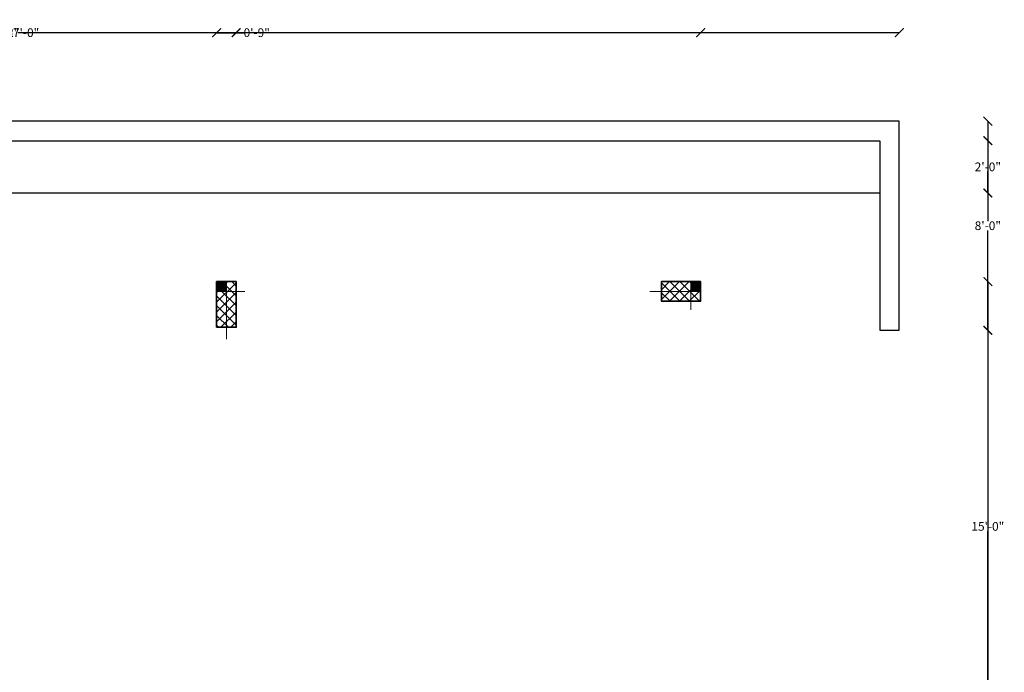
# Model space of a CAD drawing. Units: inches. Extents: x 2 to 905, y 9 to 678.
# Tile 8 of 8: x 454 to 905, y 378 to 678. Entities that reach past the tile are written whole.
import ezdxf

# ---------------------------------------------------------------- set-up
doc = ezdxf.new("R2010")
doc.units = ezdxf.units.IN
for name, color, linetype, lineweight in [('A-ANNO-DIMS', 7, 'Continuous', 18), ('A-COLS', 1, 'Continuous', 35), ('A-COLS-MARK', 1, 'Continuous', 18), ('A-COLS-MARK-PATT', 3, 'Continuous', 13), ('A-COLS-PATT', 1, 'Continuous', 13), ('C-PROP', 7, 'Continuous', 25)]:
    doc.layers.add(name, color=color, linetype=linetype, lineweight=lineweight)
doc.styles.get("Standard").update_dxf_attribs({"font": 'arial.ttf'})
doc.dimstyles.get("Standard").update_dxf_attribs({"dimtxt": 4, "dimasz": 4, "dimexe": 0.18, "dimexo": 0.0625, "dimgap": 0.09, "dimtad": 0, "dimtih": 1, "dimtoh": 1, "dimdec": 1, "dimzin": 0, "dimdsep": 46, "dimlunit": 3, "dimtxsty": 'Standard', "dimblk": 'ARCHTICK', "dimcen": 0, "dimse1": 1, "dimse2": 1, "dimclrt": 1, "dimadec": 0, "dimazin": 0, "dimtfac": 1, "dimtdec": 1, "dimtofl": 0, "dimtmove": 0, "dimatfit": 3, "dimfxl": 1, "dimtolj": 1, "dimtzin": 0, "dimarcsym": 0})

# ---------------------------------------------------------------- blocks, each defined once
blk = doc.blocks.new('COL-DATUM-R')
h = blk.add_hatch(color=256)
h.dxf.hatch_style = 1
h.paths.add_polyline_path([(13.01, 0), (13.01, 4.5), (8.51, 4.5), (8.51, 0)])
for p, q in [((8.51, 0), (8.51, 26.48)), ((13.01, 4.5), (0, 4.5))]:
    blk.add_line(p, q)
blk.add_lwpolyline([(8.51, 0), (13.01, 0), (13.01, 4.5), (8.51, 4.5)], close=True)
blk = doc.blocks.new('COL-DATUM-CROSS-SHORT')
for p, q in [((18.83, 0), (18.83, 13.01)), ((23.33, 4.5), (0, 4.5))]:
    blk.add_line(p, q)
blk = doc.blocks.new('_ArchTick')
at = {"color": 0, "linetype": 'ByBlock', "const_width": 0.15}
blk.add_lwpolyline([(-0.5, -0.5), (0.5, 0.5)], dxfattribs=at)
blk = doc.blocks.new('*D102')
at = {"layer": 'A-ANNO-DIMS', "color": 0, "lineweight": -2, "transparency": 16777216}
for p, q in [((53.05, 671.82), (448.08, 671.82)), ((857.05, 671.82), (462.03, 671.82))]:
    blk.add_line(p, q, dxfattribs=at)
at = {"layer": 'Defpoints', "color": 0, "transparency": 16777216}
for p in [(857.05, 671.82), (53.05, 631.22), (857.05, 631.22)]:
    blk.add_point(p, dxfattribs=at)
at = {"layer": 'A-ANNO-DIMS', "color": 0, "lineweight": -2, "transparency": 16777216, "xscale": 4, "yscale": 4, "zscale": 4, "rotation": 180}
blk.add_blockref('_ArchTick', (53.05, 671.82), dxfattribs=at)
at = {"layer": 'A-ANNO-DIMS', "color": 0, "lineweight": -2, "transparency": 16777216, "xscale": 4, "yscale": 4, "zscale": 4}
blk.add_blockref('_ArchTick', (857.05, 671.82), dxfattribs=at)
at = {"layer": 'A-ANNO-DIMS', "color": 1, "transparency": 16777216, "insert": (455.05, 671.82), "char_height": 4, "attachment_point": 5}
blk.add_mtext('\\A1;67\'-0"', dxfattribs=at)
blk = doc.blocks.new('*D104')
at = {"layer": 'A-ANNO-DIMS', "color": 0, "lineweight": -2, "transparency": 16777216}
for p, q in [((897.65, 535.22), (897.65, 447.35)), ((897.65, 355.22), (897.65, 443.09))]:
    blk.add_line(p, q, dxfattribs=at)
at = {"layer": 'Defpoints', "color": 0, "transparency": 16777216}
for p in [(857.05, 535.22), (897.65, 535.22), (857.05, 355.22)]:
    blk.add_point(p, dxfattribs=at)
at = {"layer": 'A-ANNO-DIMS', "color": 0, "lineweight": -2, "transparency": 16777216, "xscale": 4, "yscale": 4, "zscale": 4}
for p, rotation in [((897.65, 535.22), 90), ((897.65, 355.22), 270)]:
    blk.add_blockref('_ArchTick', p, dxfattribs=dict(at, rotation=rotation))
at = {"layer": 'A-ANNO-DIMS', "color": 1, "transparency": 16777216, "insert": (897.65, 445.22), "char_height": 4, "attachment_point": 5}
blk.add_mtext('\\A1;15\'-0"', dxfattribs=at)
blk = doc.blocks.new('*D105')
at = {"layer": 'A-ANNO-DIMS', "color": 0, "lineweight": -2, "transparency": 16777216}
for p, q in [((897.65, 631.22), (897.65, 585.35)), ((897.65, 535.22), (897.65, 581.09))]:
    blk.add_line(p, q, dxfattribs=at)
at = {"layer": 'Defpoints', "color": 0, "transparency": 16777216}
for p in [(857.05, 631.22), (897.65, 631.22), (857.05, 535.22)]:
    blk.add_point(p, dxfattribs=at)
at = {"layer": 'A-ANNO-DIMS', "color": 0, "lineweight": -2, "transparency": 16777216, "xscale": 4, "yscale": 4, "zscale": 4}
for p, rotation in [((897.65, 631.22), 90), ((897.65, 535.22), 270)]:
    blk.add_blockref('_ArchTick', p, dxfattribs=dict(at, rotation=rotation))
at = {"layer": 'A-ANNO-DIMS', "color": 1, "transparency": 16777216, "insert": (897.65, 583.22), "char_height": 4, "attachment_point": 5}
blk.add_mtext('\\A1;8\'-0"', dxfattribs=at)
blk = doc.blocks.new('*D106')
at = {"layer": 'A-ANNO-DIMS', "color": 0, "lineweight": -2, "transparency": 16777216}
for p, q in [((848.05, 14.62), (857.05, 14.62)), ((857.05, 14.62), (861.05, 14.62))]:
    blk.add_line(p, q, dxfattribs=at)
at = {"layer": 'Defpoints', "color": 0, "transparency": 16777216}
for p in [(848.05, 535.22), (857.05, 535.22), (857.05, 14.62)]:
    blk.add_point(p, dxfattribs=at)
at = {"layer": 'A-ANNO-DIMS', "color": 0, "lineweight": -2, "transparency": 16777216, "xscale": 4, "yscale": 4, "zscale": 4, "rotation": 180}
blk.add_blockref('_ArchTick', (848.05, 14.62), dxfattribs=at)
at = {"layer": 'A-ANNO-DIMS', "color": 0, "lineweight": -2, "transparency": 16777216, "xscale": 4, "yscale": 4, "zscale": 4}
blk.add_blockref('_ArchTick', (857.05, 14.62), dxfattribs=at)
at = {"layer": 'A-ANNO-DIMS', "color": 1, "transparency": 16777216, "insert": (866.46, 14.62), "char_height": 4, "attachment_point": 5}
blk.add_mtext('\\A1;0\'-9"', dxfattribs=at)
blk = doc.blocks.new('*D108')
at = {"layer": 'A-ANNO-DIMS', "color": 0, "lineweight": -2, "transparency": 16777216}
for p, q in [((897.65, 622.22), (897.65, 612.35)), ((897.65, 598.22), (897.65, 608.09))]:
    blk.add_line(p, q, dxfattribs=at)
at = {"layer": 'Defpoints', "color": 0, "transparency": 16777216}
for p in [(62.05, 622.22), (86.05, 598.22), (897.65, 598.22)]:
    blk.add_point(p, dxfattribs=at)
at = {"layer": 'A-ANNO-DIMS', "color": 0, "lineweight": -2, "transparency": 16777216, "xscale": 4, "yscale": 4, "zscale": 4}
for p, rotation in [((897.65, 622.22), 90), ((897.65, 598.22), 270)]:
    blk.add_blockref('_ArchTick', p, dxfattribs=dict(at, rotation=rotation))
at = {"layer": 'A-ANNO-DIMS', "color": 1, "transparency": 16777216, "insert": (897.65, 610.22), "char_height": 4, "attachment_point": 5}
blk.add_mtext('\\A1;2\'-0"', dxfattribs=at)
blk = doc.blocks.new('*D111')
at = {"layer": 'A-ANNO-DIMS', "color": 0, "lineweight": -2, "transparency": 16777216}
for p, q in [((116.43, 671.82), (429.56, 671.82)), ((765.93, 671.82), (452.8, 671.82))]:
    blk.add_line(p, q, dxfattribs=at)
at = {"layer": 'Defpoints', "color": 0, "transparency": 16777216}
for p in [(765.93, 671.82), (116.43, 557.58), (765.93, 557.58)]:
    blk.add_point(p, dxfattribs=at)
at = {"layer": 'A-ANNO-DIMS', "color": 0, "lineweight": -2, "transparency": 16777216, "xscale": 4, "yscale": 4, "zscale": 4, "rotation": 180}
blk.add_blockref('_ArchTick', (116.43, 671.82), dxfattribs=at)
at = {"layer": 'A-ANNO-DIMS', "color": 0, "lineweight": -2, "transparency": 16777216, "xscale": 4, "yscale": 4, "zscale": 4}
blk.add_blockref('_ArchTick', (765.93, 671.82), dxfattribs=at)
at = {"layer": 'A-ANNO-DIMS', "color": 1, "transparency": 16777216, "insert": (441.18, 671.82), "char_height": 4, "attachment_point": 5}
blk.add_mtext('\\A1;54\'-1 1/2"', dxfattribs=at)
blk = doc.blocks.new('*D112')
at = {"layer": 'A-ANNO-DIMS', "color": 0, "lineweight": -2, "transparency": 16777216}
for p, q in [((897.65, 557.58), (897.65, 345.21)), ((897.65, 128.58), (897.65, 340.94))]:
    blk.add_line(p, q, dxfattribs=at)
at = {"layer": 'Defpoints', "color": 0, "transparency": 16777216}
for p in [(417.93, 557.58), (897.65, 557.58), (417.93, 128.58)]:
    blk.add_point(p, dxfattribs=at)
at = {"layer": 'A-ANNO-DIMS', "color": 0, "lineweight": -2, "transparency": 16777216, "xscale": 4, "yscale": 4, "zscale": 4}
for p, rotation in [((897.65, 557.58), 90), ((897.65, 128.58), 270)]:
    blk.add_blockref('_ArchTick', p, dxfattribs=dict(at, rotation=rotation))
at = {"layer": 'A-ANNO-DIMS', "color": 1, "transparency": 16777216, "insert": (897.65, 343.08), "char_height": 4, "attachment_point": 5}
blk.add_mtext('\\A1;35\'-9"', dxfattribs=at)
blk = doc.blocks.new('*D117')
at = {"layer": 'A-ANNO-DIMS', "color": 0, "lineweight": -2, "transparency": 16777216}
for p, q in [((543.93, 671.82), (552.93, 671.82)), ((552.93, 671.82), (556.93, 671.82))]:
    blk.add_line(p, q, dxfattribs=at)
at = {"layer": 'Defpoints', "color": 0, "transparency": 16777216}
for p in [(552.93, 671.82), (543.93, 149.58), (552.93, 149.58)]:
    blk.add_point(p, dxfattribs=at)
at = {"layer": 'A-ANNO-DIMS', "color": 0, "lineweight": -2, "transparency": 16777216, "xscale": 4, "yscale": 4, "zscale": 4, "rotation": 180}
blk.add_blockref('_ArchTick', (543.93, 671.82), dxfattribs=at)
at = {"layer": 'A-ANNO-DIMS', "color": 0, "lineweight": -2, "transparency": 16777216, "xscale": 4, "yscale": 4, "zscale": 4}
blk.add_blockref('_ArchTick', (552.93, 671.82), dxfattribs=at)
at = {"layer": 'A-ANNO-DIMS', "color": 1, "transparency": 16777216, "insert": (562.34, 671.82), "char_height": 4, "attachment_point": 5}
blk.add_mtext('\\A1;0\'-9"', dxfattribs=at)
blk = doc.blocks.new('*D119')
at = {"layer": 'A-ANNO-DIMS', "color": 0, "lineweight": -2, "transparency": 16777216}
for p, q in [((747.93, 14.62), (751.72, 14.62)), ((765.93, 14.62), (762.15, 14.62))]:
    blk.add_line(p, q, dxfattribs=at)
at = {"layer": 'Defpoints', "color": 0, "transparency": 16777216}
for p in [(747.93, 548.58), (765.93, 548.58), (765.93, 14.62)]:
    blk.add_point(p, dxfattribs=at)
at = {"layer": 'A-ANNO-DIMS', "color": 0, "lineweight": -2, "transparency": 16777216, "xscale": 4, "yscale": 4, "zscale": 4, "rotation": 180}
blk.add_blockref('_ArchTick', (747.93, 14.62), dxfattribs=at)
at = {"layer": 'A-ANNO-DIMS', "color": 0, "lineweight": -2, "transparency": 16777216, "xscale": 4, "yscale": 4, "zscale": 4}
blk.add_blockref('_ArchTick', (765.93, 14.62), dxfattribs=at)
at = {"layer": 'A-ANNO-DIMS', "color": 1, "transparency": 16777216, "insert": (756.93, 14.62), "char_height": 4, "attachment_point": 5}
blk.add_mtext('\\A1;1\'-6"', dxfattribs=at)

msp = doc.modelspace()

# ---------------------------------------------------------------- hatches: boundary and pattern name
at = {"layer": 'A-COLS-MARK-PATT'}
h = msp.add_hatch(color=256, dxfattribs=at)
h.dxf.hatch_style = 1
h.paths.add_polyline_path([(765.93, 557.58), (761.43, 557.58), (761.43, 553.08), (765.93, 553.08)])
at = {"layer": 'A-COLS-PATT'}
h = msp.add_hatch(dxfattribs=at)
h.set_pattern_fill('ANSI37', color=256, angle=-180)
h.set_pattern_definition([(225, (-408.7418, 893.045), (2.245064, -2.245064), []), (315, (-408.7418, 893.045), (2.245064, 2.245064), [])])
h.paths.add_polyline_path([(552.93, 553.08), (548.43, 553.08), (548.43, 557.58), (552.93, 557.58)])
h.paths.add_polyline_path([(552.93, 536.58), (548.43, 536.58), (548.43, 553.08), (552.93, 553.08)])
h.paths.add_polyline_path([(548.43, 536.58), (543.93, 536.58), (543.93, 553.08), (548.43, 553.08)])
h = msp.add_hatch(dxfattribs=at)
h.set_pattern_fill('ANSI37', color=256, angle=90)
h.set_pattern_definition([(135, (1041.4012, 645.212), (-2.245064, -2.245064), []), (225, (1041.4012, 645.212), (2.245064, -2.245064), [])])
h.paths.add_polyline_path([(761.43, 548.58), (761.43, 553.08), (765.93, 553.08), (765.93, 548.58)])
h.paths.add_polyline_path([(747.98, 557.58), (747.98, 553.08), (761.43, 553.08), (761.43, 557.58)])
h.paths.add_polyline_path([(747.98, 553.08), (747.98, 548.58), (761.43, 548.58), (761.43, 553.08)])

# ---------------------------------------------------------------- linework, layer by layer
at = {"layer": 'A-COLS'}
msp.add_line((747.93, 548.58), (747.93, 557.58), dxfattribs=at)
for points in [[(543.93, 536.58), (552.93, 536.58), (552.93, 557.58), (543.93, 557.58)], [(747.93, 548.58), (756.93, 548.58), (765.93, 548.58), (765.93, 557.58), (747.93, 557.58)], [(747.98, 557.58), (747.98, 548.58), (765.93, 548.58), (765.93, 557.58)]]:
    msp.add_lwpolyline(points, close=True, dxfattribs=at)
at = {"layer": 'A-COLS-MARK'}
msp.add_lwpolyline([(765.93, 553.08), (765.93, 557.58), (761.43, 557.58), (761.43, 553.08)], close=True, dxfattribs=at)
at = {"layer": 'C-PROP'}
msp.add_lwpolyline([(857.05, 535.22), (857.05, 631.22), (53.05, 631.22), (53.05, 55.22), (857.05, 55.22), (857.05, 355.22), (848.05, 355.22), (848.05, 64.22), (62.05, 64.22), (62.05, 622.22), (848.05, 622.22), (848.05, 535.22)], close=True, dxfattribs=at)
msp.add_lwpolyline([(848.05, 598.22), (86.05, 598.22), (86.05, 88.22), (824.05, 88.22), (824.05, 355.22), (836.05, 355.22), (848.05, 355.22)], dxfattribs=at)

# ---------------------------------------------------------------- block references
at = {"layer": 'A-COLS-MARK', "rotation": 180}
msp.add_blockref('COL-DATUM-R', (556.94, 557.58), dxfattribs=at)
at = {"layer": 'A-COLS-MARK', "extrusion": (0, 0, -1), "zscale": -1, "rotation": 180}
msp.add_blockref('COL-DATUM-CROSS-SHORT', (-742.6, 557.58), dxfattribs=at)

# ---------------------------------------------------------------- dimensions: what is measured, and where the dimension line sits
at = {"layer": 'A-ANNO-DIMS'}
for base, p1, p2, picture, middle in [((765.93, 671.82), (116.43, 557.58), (765.93, 557.58), '*D111', (441.18, 671.82)), ((857.05, 671.82), (53.05, 631.22), (857.05, 631.22), '*D102', (455.05, 671.82)), ((552.93, 671.82), (543.93, 149.58), (552.93, 149.58), '*D117', (562.34, 671.82)), ((765.93, 14.62), (747.93, 548.58), (765.93, 548.58), '*D119', (756.93, 14.62)), ((857.05, 14.62), (848.05, 535.22), (857.05, 535.22), '*D106', (866.46, 14.62))]:
    dim = msp.add_linear_dim(base=base, p1=p1, p2=p2, dimstyle='Standard', override={"dimdec": 1, "dimlfac": 1, "dimrnd": 0, "dimzin": 1, "dimdsep": 46, "dimlunit": 4, "dimfrac": 2}, dxfattribs=at)
    dim.commit()
    dim.dimension.update_dxf_attribs({"geometry": picture, "text_midpoint": middle})
for base, p1, p2, picture, middle in [((897.65, 631.22), (857.05, 535.22), (857.05, 631.22), '*D105', (897.65, 583.22)), ((897.65, 598.22), (62.05, 622.22), (86.05, 598.22), '*D108', (897.65, 610.22)), ((897.65, 557.58), (417.93, 128.58), (417.93, 557.58), '*D112', (897.65, 343.08)), ((897.65, 535.22), (857.05, 355.22), (857.05, 535.22), '*D104', (897.65, 445.22))]:
    dim = msp.add_linear_dim(base=base, p1=p1, p2=p2, angle=90, dimstyle='Standard', override={"dimdec": 1, "dimlfac": 1, "dimrnd": 0, "dimzin": 1, "dimdsep": 46, "dimlunit": 4, "dimfrac": 2}, dxfattribs=at)
    dim.commit()
    dim.dimension.update_dxf_attribs({"geometry": picture, "text_midpoint": middle})

doc.saveas('drawing.dxf')
